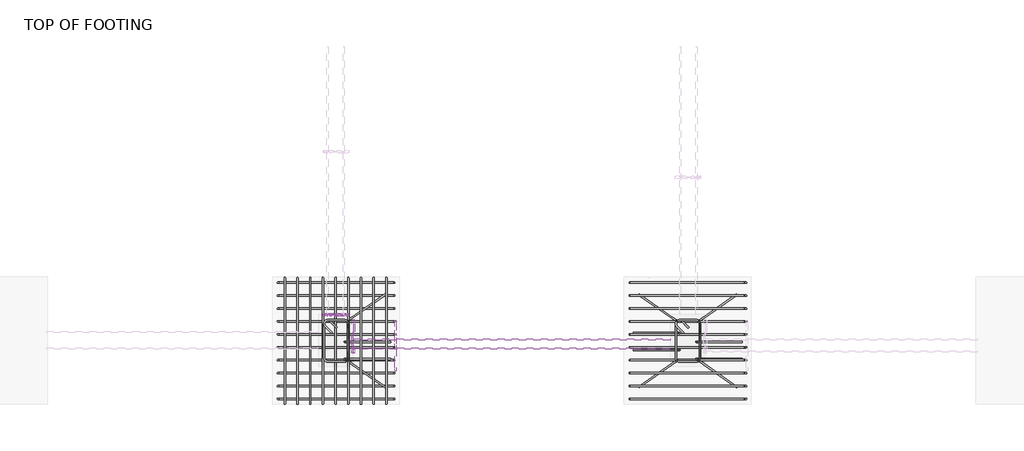
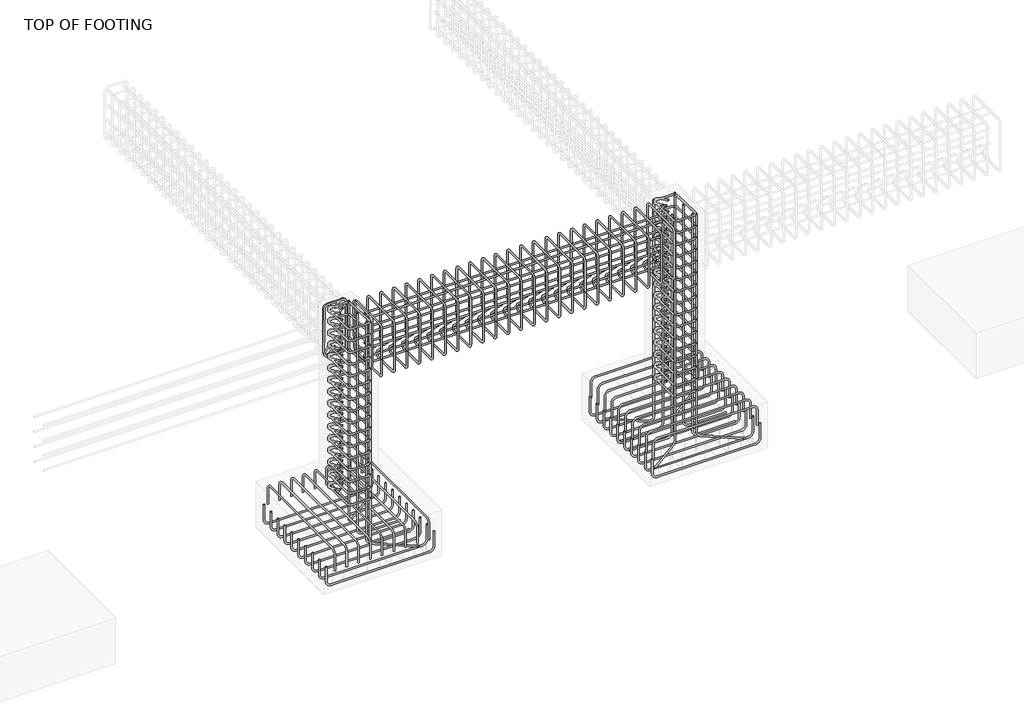
# One storey, part 3 of 18: 21 reinforcing bars.
"""IFC4 building model written with IfcOpenShell, lengths in millimetres."""

from ifc_helpers import new_model, si_unit, point, frame, origin, place, context, project, spatial, polyline, circle_curve, trimmed, segment, composite_curve, source, transform, mapped, element, save
from ifc_brep_helpers import swept_disk

model = new_model("IFC4")

# Units and contexts
model_context = context("Model", 3, world=origin())
ifc_project = project(units=[si_unit("LENGTHUNIT", "METRE", prefix="MILLI")], contexts=[model_context])

# Site, building, storey
site = spatial("IfcSite", under=ifc_project)
building = spatial("IfcBuilding", under=site)
storey = spatial("IfcBuildingStorey", under=building, Name="TOP OF FOOTING", Elevation=-1828.8)

# Reinforcing bars
placement = place(None, origin())
reinforcing_bar_shape = source(origin(), model_context, "Body", "SolidModel", [
    swept_disk(composite_curve([segment(polyline([(-7988.6954038, 5770.3841028, -1782.45), (-8044.4389667, 5826.1276657, -1782.45)]), True, "CONTINUOUS"), segment(trimmed(circle_curve(frame((-8066.6067643, 5803.9598681, -1782.45), z_axis=(0.0, 0.0, 1.0), x_axis=(22.167797600000085, 22.167797600000085, 0.0)), 31.35), [point((-8044.4389667, 5826.1276657, -1782.45))], [point((-8097.9567643, 5803.9598681, -1782.45))], True, "CARTESIAN"), True, "CONTINUOUS"), segment(polyline([(-8097.9567643, 5803.9598681, -1782.45), (-8097.9567643, 5509.3598681, -1782.45)]), True, "CONTINUOUS"), segment(trimmed(circle_curve(frame((-8066.6067643, 5509.3598681, -1782.45), z_axis=(0.0, 0.0, 1.0), x_axis=(-31.350000000000364, 0.0, 0.0)), 31.35), [point((-8097.9567643, 5509.3598681, -1782.45))], [point((-8066.6067643, 5478.0098681, -1782.45))], True, "CARTESIAN"), True, "CONTINUOUS"), segment(polyline([(-8066.6067643, 5478.0098681, -1782.45), (-7922.0067643, 5478.0098681, -1782.45)]), True, "CONTINUOUS"), segment(trimmed(circle_curve(frame((-7922.0067643, 5509.3400831, -1783.5636125), z_axis=(0.0, 0.03552192833448201, 0.9993688971583016), x_axis=(0.0, -31.330214999999953, 1.1136125000000447)), 31.35), [point((-7922.0067643, 5478.0098681, -1782.45))], [point((-7890.6567643, 5509.3400831, -1783.5636125))], True, "CARTESIAN"), True, "CONTINUOUS"), segment(polyline([(-7890.6567643, 5509.3400831, -1783.5636125), (-7890.6567643, 5803.9796532, -1794.0363875)]), True, "CONTINUOUS"), segment(trimmed(circle_curve(frame((-7922.0067643, 5803.9796532, -1794.0363875), z_axis=(0.0, 0.03552192833448201, 0.9993688971583016), x_axis=(31.350000000000364, 0.0, 0.0)), 31.35), [point((-7890.6567643, 5803.9796532, -1794.0363875))], [point((-7922.0067643, 5835.3098681, -1795.15))], True, "CARTESIAN"), True, "CONTINUOUS"), segment(polyline([(-7922.0067643, 5835.3098681, -1795.15), (-8066.6067643, 5835.3098681, -1795.15)]), True, "CONTINUOUS"), segment(trimmed(circle_curve(frame((-8066.6067643, 5803.9598681, -1795.15), z_axis=(0.0, 0.0, 1.0), x_axis=(0.0, 31.350000000000364, 0.0)), 31.35), [point((-8066.6067643, 5835.3098681, -1795.15))], [point((-8088.7745619, 5781.7920705, -1795.15))], True, "CARTESIAN"), True, "CONTINUOUS"), segment(polyline([(-8088.7745619, 5781.7920705, -1795.15), (-8033.030999, 5726.0485076, -1795.15)]), True, "CONTINUOUS")], self_intersect=False), 6.35),
])
element("IfcReinforcingBar", 1, at=placement, inside=storey, context=model_context, shape_type="MappedRepresentation", body=[
    mapped(reinforcing_bar_shape, transform((0.0, 0.0, 0.0), x_axis=(1.0, 0.0, 0.0), y_axis=(0.0, 1.0, 0.0), z_axis=(0.0, 0.0, 1.0))),
    mapped(reinforcing_bar_shape, transform((0.0, 0.0, 116.0092918), x_axis=(1.0, 0.0, 0.0), y_axis=(0.0, 1.0, 0.0), z_axis=(0.0, 0.0, 1.0))),
    mapped(reinforcing_bar_shape, transform((0.0, 0.0, 232.0185836), x_axis=(1.0, 0.0, 0.0), y_axis=(0.0, 1.0, 0.0), z_axis=(0.0, 0.0, 1.0))),
    mapped(reinforcing_bar_shape, transform((0.0, 0.0, 348.0278755), x_axis=(1.0, 0.0, 0.0), y_axis=(0.0, 1.0, 0.0), z_axis=(0.0, 0.0, 1.0))),
    mapped(reinforcing_bar_shape, transform((0.0, 0.0, 464.0371673), x_axis=(1.0, 0.0, 0.0), y_axis=(0.0, 1.0, 0.0), z_axis=(0.0, 0.0, 1.0))),
    mapped(reinforcing_bar_shape, transform((0.0, 0.0, 580.0464591), x_axis=(1.0, 0.0, 0.0), y_axis=(0.0, 1.0, 0.0), z_axis=(0.0, 0.0, 1.0))),
    mapped(reinforcing_bar_shape, transform((0.0, 0.0, 696.0557509), x_axis=(1.0, 0.0, 0.0), y_axis=(0.0, 1.0, 0.0), z_axis=(0.0, 0.0, 1.0))),
    mapped(reinforcing_bar_shape, transform((0.0, 0.0, 812.0650428), x_axis=(1.0, 0.0, 0.0), y_axis=(0.0, 1.0, 0.0), z_axis=(0.0, 0.0, 1.0))),
    mapped(reinforcing_bar_shape, transform((0.0, 0.0, 928.0743346), x_axis=(1.0, 0.0, 0.0), y_axis=(0.0, 1.0, 0.0), z_axis=(0.0, 0.0, 1.0))),
    mapped(reinforcing_bar_shape, transform((0.0, 0.0, 1044.0836264), x_axis=(1.0, 0.0, 0.0), y_axis=(0.0, 1.0, 0.0), z_axis=(0.0, 0.0, 1.0))),
    mapped(reinforcing_bar_shape, transform((0.0, 0.0, 1160.0929182), x_axis=(1.0, 0.0, 0.0), y_axis=(0.0, 1.0, 0.0), z_axis=(0.0, 0.0, 1.0))),
    mapped(reinforcing_bar_shape, transform((0.0, 0.0, 1276.1022101), x_axis=(1.0, 0.0, 0.0), y_axis=(0.0, 1.0, 0.0), z_axis=(0.0, 0.0, 1.0))),
    mapped(reinforcing_bar_shape, transform((0.0, 0.0, 1392.1115019), x_axis=(1.0, 0.0, 0.0), y_axis=(0.0, 1.0, 0.0), z_axis=(0.0, 0.0, 1.0))),
    mapped(reinforcing_bar_shape, transform((0.0, 0.0, 1508.1207937), x_axis=(1.0, 0.0, 0.0), y_axis=(0.0, 1.0, 0.0), z_axis=(0.0, 0.0, 1.0))),
    mapped(reinforcing_bar_shape, transform((0.0, 0.0, 1624.1300855), x_axis=(1.0, 0.0, 0.0), y_axis=(0.0, 1.0, 0.0), z_axis=(0.0, 0.0, 1.0))),
    mapped(reinforcing_bar_shape, transform((0.0, 0.0, 1740.1393774), x_axis=(1.0, 0.0, 0.0), y_axis=(0.0, 1.0, 0.0), z_axis=(0.0, 0.0, 1.0))),
])
element("IfcReinforcingBar", 2, at=placement, inside=storey, context=model_context, shape_type="SolidModel", body=[
    swept_disk(composite_curve([segment(polyline([(-7895.6275643, 5830.3098681, -40.0), (-7895.6275643, 5830.3098681, -2185.2530621)]), True, "CONTINUOUS"), segment(trimmed(circle_curve(frame((-7857.6598671, 5856.895136, -2185.2530621), z_axis=(0.5735764363510552, -0.8191520442889855, 0.0), x_axis=(-37.96769719999975, -26.585267899999963, 0.0)), 46.35), [point((-7895.6275643, 5830.3098681, -2185.2530621))], [point((-7857.6598671, 5856.895136, -2231.6030621))], True, "CARTESIAN"), True, "CONTINUOUS"), segment(polyline([(-7857.6598671, 5856.895136, -2231.6030621), (-7569.9927964, 6058.3217874, -2231.6030621)]), True, "CONTINUOUS")], self_intersect=False), 6.35),
])
element("IfcReinforcingBar", 3, at=placement, inside=storey, context=model_context, shape_type="SolidModel", body=[
    swept_disk(composite_curve([segment(polyline([(-7895.6275643, 5483.0098681, -40.0), (-7895.6275643, 5483.0098681, -2185.2530621)]), True, "CONTINUOUS"), segment(trimmed(circle_curve(frame((-7857.6598671, 5456.4246003, -2185.2530621), z_axis=(-0.5735764363510997, -0.8191520442889543, 0.0), x_axis=(-37.96769719999975, 26.58526780000011, 0.0)), 46.35), [point((-7895.6275643, 5483.0098681, -2185.2530621))], [point((-7857.6598671, 5456.4246003, -2231.6030621))], True, "CARTESIAN"), True, "CONTINUOUS"), segment(polyline([(-7857.6598671, 5456.4246003, -2231.6030621), (-7569.9927964, 5254.9979489, -2231.6030621)]), True, "CONTINUOUS")], self_intersect=False), 6.35),
])
reinforcing_bar_2_shape = source(origin(), model_context, "Body", "SolidModel", [
    swept_disk(composite_curve([segment(polyline([(-7920.6275643, 5499.8477614, -40.0), (-7920.6275643, 5499.8477614, -2185.2530621)]), True, "CONTINUOUS"), segment(trimmed(circle_curve(frame((-7874.2775643, 5499.8477614, -2185.2530621), z_axis=(0.0, -1.0, 0.0), x_axis=(-46.349999999999454, 0.0, 0.0)), 46.35), [point((-7920.6275643, 5499.8477614, -2185.2530621))], [point((-7874.2775643, 5499.8477614, -2231.6030621))], True, "CARTESIAN"), True, "CONTINUOUS"), segment(polyline([(-7874.2775643, 5499.8477614, -2231.6030621), (-7523.1009144, 5499.8477614, -2231.6030621)]), True, "CONTINUOUS")], self_intersect=False), 6.35),
])
element("IfcReinforcingBar", 4, at=placement, inside=storey, context=model_context, shape_type="MappedRepresentation", body=[
    mapped(reinforcing_bar_2_shape, transform((0.0, 0.0, 0.0), x_axis=(1.0, 0.0, 0.0), y_axis=(0.0, 1.0, 0.0), z_axis=(0.0, 0.0, 1.0))),
    mapped(reinforcing_bar_2_shape, transform((0.0, 148.3194112, 0.0), x_axis=(1.0, 0.0, 0.0), y_axis=(0.0, 1.0, 0.0), z_axis=(0.0, 0.0, 1.0))),
])
reinforcing_bar_3_shape = source(origin(), model_context, "Body", "SolidModel", [
    swept_disk(composite_curve([segment(polyline([(-5019.9859643, 5574.8477614, -40.0), (-5019.9859643, 5574.8477614, -2185.2530621)]), True, "CONTINUOUS"), segment(trimmed(circle_curve(frame((-5066.3359643, 5574.8477614, -2185.2530621), z_axis=(0.0, 1.0, 0.0), x_axis=(46.350000000000364, 0.0, 0.0)), 46.35), [point((-5019.9859643, 5574.8477614, -2185.2530621))], [point((-5066.3359643, 5574.8477614, -2231.6030621))], True, "CARTESIAN"), True, "CONTINUOUS"), segment(polyline([(-5066.3359643, 5574.8477614, -2231.6030621), (-5417.5126143, 5574.8477614, -2231.6030621)]), True, "CONTINUOUS")], self_intersect=False), 6.35),
])
element("IfcReinforcingBar", 5, at=placement, inside=storey, context=model_context, shape_type="MappedRepresentation", body=[
    mapped(reinforcing_bar_3_shape, transform((0.0, 0.0, 0.0), x_axis=(1.0, 0.0, 0.0), y_axis=(0.0, 1.0, 0.0), z_axis=(0.0, 0.0, 1.0))),
    mapped(reinforcing_bar_3_shape, transform((0.0, 148.3194112, 0.0), x_axis=(1.0, 0.0, 0.0), y_axis=(0.0, 1.0, 0.0), z_axis=(0.0, 0.0, 1.0))),
])
element("IfcReinforcingBar", 6, at=placement, inside=storey, context=model_context, shape_type="SolidModel", body=[
    swept_disk(composite_curve([segment(polyline([(-5044.9859643, 5830.3098681, -40.0), (-5044.9859643, 5830.3098681, -2185.2530621)]), True, "CONTINUOUS"), segment(trimmed(circle_curve(frame((-5082.9536616, 5856.895136, -2185.2530621), z_axis=(0.5735764363510552, 0.8191520442889856, 0.0), x_axis=(37.9676972999996, -26.585267899999963, 0.0)), 46.35), [point((-5044.9859643, 5830.3098681, -2185.2530621))], [point((-5082.9536616, 5856.895136, -2231.6030621))], True, "CARTESIAN"), True, "CONTINUOUS"), segment(polyline([(-5082.9536616, 5856.895136, -2231.6030621), (-5370.6207323, 6058.3217874, -2231.6030621)]), True, "CONTINUOUS")], self_intersect=False), 6.35),
])
reinforcing_bar_4_shape = source(origin(), model_context, "Body", "SolidModel", [
    swept_disk(composite_curve([segment(polyline([(-4940.6954038, 5770.3841028, -1782.45), (-4996.4389667, 5826.1276657, -1782.45)]), True, "CONTINUOUS"), segment(trimmed(circle_curve(frame((-5018.6067643, 5803.9598681, -1782.45), z_axis=(0.0, 0.0, 1.0), x_axis=(22.167797600000085, 22.167797600000085, 0.0)), 31.35), [point((-4996.4389667, 5826.1276657, -1782.45))], [point((-5049.9567643, 5803.9598681, -1782.45))], True, "CARTESIAN"), True, "CONTINUOUS"), segment(polyline([(-5049.9567643, 5803.9598681, -1782.45), (-5049.9567643, 5509.3598681, -1782.45)]), True, "CONTINUOUS"), segment(trimmed(circle_curve(frame((-5018.6067643, 5509.3598681, -1782.45), z_axis=(0.0, 0.0, 1.0), x_axis=(-31.350000000000364, 0.0, 0.0)), 31.35), [point((-5049.9567643, 5509.3598681, -1782.45))], [point((-5018.6067643, 5478.0098681, -1782.45))], True, "CARTESIAN"), True, "CONTINUOUS"), segment(polyline([(-5018.6067643, 5478.0098681, -1782.45), (-4874.0067643, 5478.0098681, -1782.45)]), True, "CONTINUOUS"), segment(trimmed(circle_curve(frame((-4874.0067643, 5509.3400831, -1783.5636125), z_axis=(0.0, 0.0355219283344819, 0.9993688971583016), x_axis=(0.0, -31.330214999999953, 1.1136125000000447)), 31.35), [point((-4874.0067643, 5478.0098681, -1782.45))], [point((-4842.6567643, 5509.3400831, -1783.5636125))], True, "CARTESIAN"), True, "CONTINUOUS"), segment(polyline([(-4842.6567643, 5509.3400831, -1783.5636125), (-4842.6567643, 5803.9796532, -1794.0363875)]), True, "CONTINUOUS"), segment(trimmed(circle_curve(frame((-4874.0067643, 5803.9796532, -1794.0363875), z_axis=(0.0, 0.0355219283344819, 0.9993688971583016), x_axis=(31.350000000000364, 0.0, 0.0)), 31.35), [point((-4842.6567643, 5803.9796532, -1794.0363875))], [point((-4874.0067643, 5835.3098681, -1795.15))], True, "CARTESIAN"), True, "CONTINUOUS"), segment(polyline([(-4874.0067643, 5835.3098681, -1795.15), (-5018.6067643, 5835.3098681, -1795.15)]), True, "CONTINUOUS"), segment(trimmed(circle_curve(frame((-5018.6067643, 5803.9598681, -1795.15), z_axis=(0.0, 0.0, 1.0), x_axis=(0.0, 31.350000000000364, 0.0)), 31.35), [point((-5018.6067643, 5835.3098681, -1795.15))], [point((-5040.7745619, 5781.7920705, -1795.15))], True, "CARTESIAN"), True, "CONTINUOUS"), segment(polyline([(-5040.7745619, 5781.7920705, -1795.15), (-4985.030999, 5726.0485076, -1795.15)]), True, "CONTINUOUS")], self_intersect=False), 6.35),
])
element("IfcReinforcingBar", 7, at=placement, inside=storey, context=model_context, shape_type="MappedRepresentation", body=[
    mapped(reinforcing_bar_4_shape, transform((0.0, 0.0, 0.0), x_axis=(1.0, 0.0, 0.0), y_axis=(0.0, 1.0, 0.0), z_axis=(0.0, 0.0, 1.0))),
    mapped(reinforcing_bar_4_shape, transform((0.0, 0.0, 116.0092918), x_axis=(1.0, 0.0, 0.0), y_axis=(0.0, 1.0, 0.0), z_axis=(0.0, 0.0, 1.0))),
    mapped(reinforcing_bar_4_shape, transform((0.0, 0.0, 232.0185836), x_axis=(1.0, 0.0, 0.0), y_axis=(0.0, 1.0, 0.0), z_axis=(0.0, 0.0, 1.0))),
    mapped(reinforcing_bar_4_shape, transform((0.0, 0.0, 348.0278755), x_axis=(1.0, 0.0, 0.0), y_axis=(0.0, 1.0, 0.0), z_axis=(0.0, 0.0, 1.0))),
    mapped(reinforcing_bar_4_shape, transform((0.0, 0.0, 464.0371673), x_axis=(1.0, 0.0, 0.0), y_axis=(0.0, 1.0, 0.0), z_axis=(0.0, 0.0, 1.0))),
    mapped(reinforcing_bar_4_shape, transform((0.0, 0.0, 580.0464591), x_axis=(1.0, 0.0, 0.0), y_axis=(0.0, 1.0, 0.0), z_axis=(0.0, 0.0, 1.0))),
    mapped(reinforcing_bar_4_shape, transform((0.0, 0.0, 696.0557509), x_axis=(1.0, 0.0, 0.0), y_axis=(0.0, 1.0, 0.0), z_axis=(0.0, 0.0, 1.0))),
    mapped(reinforcing_bar_4_shape, transform((0.0, 0.0, 812.0650428), x_axis=(1.0, 0.0, 0.0), y_axis=(0.0, 1.0, 0.0), z_axis=(0.0, 0.0, 1.0))),
    mapped(reinforcing_bar_4_shape, transform((0.0, 0.0, 928.0743346), x_axis=(1.0, 0.0, 0.0), y_axis=(0.0, 1.0, 0.0), z_axis=(0.0, 0.0, 1.0))),
    mapped(reinforcing_bar_4_shape, transform((0.0, 0.0, 1044.0836264), x_axis=(1.0, 0.0, 0.0), y_axis=(0.0, 1.0, 0.0), z_axis=(0.0, 0.0, 1.0))),
    mapped(reinforcing_bar_4_shape, transform((0.0, 0.0, 1160.0929182), x_axis=(1.0, 0.0, 0.0), y_axis=(0.0, 1.0, 0.0), z_axis=(0.0, 0.0, 1.0))),
    mapped(reinforcing_bar_4_shape, transform((0.0, 0.0, 1276.1022101), x_axis=(1.0, 0.0, 0.0), y_axis=(0.0, 1.0, 0.0), z_axis=(0.0, 0.0, 1.0))),
    mapped(reinforcing_bar_4_shape, transform((0.0, 0.0, 1392.1115019), x_axis=(1.0, 0.0, 0.0), y_axis=(0.0, 1.0, 0.0), z_axis=(0.0, 0.0, 1.0))),
    mapped(reinforcing_bar_4_shape, transform((0.0, 0.0, 1508.1207937), x_axis=(1.0, 0.0, 0.0), y_axis=(0.0, 1.0, 0.0), z_axis=(0.0, 0.0, 1.0))),
    mapped(reinforcing_bar_4_shape, transform((0.0, 0.0, 1624.1300855), x_axis=(1.0, 0.0, 0.0), y_axis=(0.0, 1.0, 0.0), z_axis=(0.0, 0.0, 1.0))),
    mapped(reinforcing_bar_4_shape, transform((0.0, 0.0, 1740.1393774), x_axis=(1.0, 0.0, 0.0), y_axis=(0.0, 1.0, 0.0), z_axis=(0.0, 0.0, 1.0))),
])
element("IfcReinforcingBar", 8, at=placement, inside=storey, context=model_context, shape_type="SolidModel", body=[
    swept_disk(composite_curve([segment(polyline([(-4847.6275643, 5830.3098681, -40.0), (-4847.6275643, 5830.3098681, -2185.2530621)]), True, "CONTINUOUS"), segment(trimmed(circle_curve(frame((-4809.6598671, 5856.895136, -2185.2530621), z_axis=(0.5735764363510553, -0.8191520442889855, 0.0), x_axis=(-37.96769719999975, -26.585267899999963, 0.0)), 46.35), [point((-4847.6275643, 5830.3098681, -2185.2530621))], [point((-4809.6598671, 5856.895136, -2231.6030621))], True, "CARTESIAN"), True, "CONTINUOUS"), segment(polyline([(-4809.6598671, 5856.895136, -2231.6030621), (-4521.9927964, 6058.3217874, -2231.6030621)]), True, "CONTINUOUS")], self_intersect=False), 6.35),
])
element("IfcReinforcingBar", 9, at=placement, inside=storey, context=model_context, shape_type="SolidModel", body=[
    swept_disk(composite_curve([segment(polyline([(-5044.9859643, 5483.0098681, -40.0), (-5044.9859643, 5483.0098681, -2185.2530621)]), True, "CONTINUOUS"), segment(trimmed(circle_curve(frame((-5082.9536616, 5456.4246003, -2185.2530621), z_axis=(-0.5735764363510106, 0.8191520442890168, 0.0), x_axis=(37.9676972999996, 26.58526780000011, 0.0)), 46.35), [point((-5044.9859643, 5483.0098681, -2185.2530621))], [point((-5082.9536616, 5456.4246003, -2231.6030621))], True, "CARTESIAN"), True, "CONTINUOUS"), segment(polyline([(-5082.9536616, 5456.4246003, -2231.6030621), (-5370.6207323, 5254.9979489, -2231.6030621)]), True, "CONTINUOUS")], self_intersect=False), 6.35),
])
element("IfcReinforcingBar", 10, at=placement, inside=storey, context=model_context, shape_type="SolidModel", body=[
    swept_disk(composite_curve([segment(polyline([(-4847.6275643, 5483.0098681, -40.0), (-4847.6275643, 5483.0098681, -2185.2530621)]), True, "CONTINUOUS"), segment(trimmed(circle_curve(frame((-4809.6598671, 5456.4246003, -2185.2530621), z_axis=(-0.5735764363510997, -0.8191520442889544, 0.0), x_axis=(-37.96769719999975, 26.58526780000011, 0.0)), 46.35), [point((-4847.6275643, 5483.0098681, -2185.2530621))], [point((-4809.6598671, 5456.4246003, -2231.6030621))], True, "CARTESIAN"), True, "CONTINUOUS"), segment(polyline([(-4809.6598671, 5456.4246003, -2231.6030621), (-4521.9927964, 5254.9979489, -2231.6030621)]), True, "CONTINUOUS")], self_intersect=False), 6.35),
])
reinforcing_bar_5_shape = source(origin(), model_context, "Body", "SolidModel", [
    swept_disk(composite_curve([segment(polyline([(-4872.6275643, 5499.8477614, -40.0), (-4872.6275643, 5499.8477614, -2185.2530621)]), True, "CONTINUOUS"), segment(trimmed(circle_curve(frame((-4826.2775643, 5499.8477614, -2185.2530621), z_axis=(0.0, -1.0, 0.0), x_axis=(-46.349999999999454, 0.0, 0.0)), 46.35), [point((-4872.6275643, 5499.8477614, -2185.2530621))], [point((-4826.2775643, 5499.8477614, -2231.6030621))], True, "CARTESIAN"), True, "CONTINUOUS"), segment(polyline([(-4826.2775643, 5499.8477614, -2231.6030621), (-4475.1009144, 5499.8477614, -2231.6030621)]), True, "CONTINUOUS")], self_intersect=False), 6.35),
])
element("IfcReinforcingBar", 11, at=placement, inside=storey, context=model_context, shape_type="MappedRepresentation", body=[
    mapped(reinforcing_bar_5_shape, transform((0.0, 0.0, 0.0), x_axis=(1.0, 0.0, 0.0), y_axis=(0.0, 1.0, 0.0), z_axis=(0.0, 0.0, 1.0))),
    mapped(reinforcing_bar_5_shape, transform((0.0, 148.3194112, 0.0), x_axis=(1.0, 0.0, 0.0), y_axis=(0.0, 1.0, 0.0), z_axis=(0.0, 0.0, 1.0))),
])
reinforcing_bar_6_shape = source(origin(), model_context, "Body", "SolidModel", [
    swept_disk(composite_curve([segment(polyline([(-4442.6567643, 6160.3098681, -2046.8654906), (-4442.6567643, 6160.3098681, -2194.1654906)]), True, "CONTINUOUS"), segment(trimmed(circle_curve(frame((-4489.0067643, 6160.3098681, -2194.1654906), z_axis=(0.0, 1.0, 0.0), x_axis=(46.350000000000364, 0.0, 0.0)), 46.35), [point((-4442.6567643, 6160.3098681, -2194.1654906))], [point((-4489.0067643, 6160.3098681, -2240.5154906))], True, "CARTESIAN"), True, "CONTINUOUS"), segment(polyline([(-4489.0067643, 6160.3098681, -2240.5154906), (-5403.6067643, 6160.3098681, -2240.5154906)]), True, "CONTINUOUS"), segment(trimmed(circle_curve(frame((-5403.6067643, 6160.3098681, -2194.1654906), z_axis=(0.0, 1.0, 0.0), x_axis=(0.0, 0.0, -46.34999999999991)), 46.35), [point((-5403.6067643, 6160.3098681, -2240.5154906))], [point((-5449.9567643, 6160.3098681, -2194.1654906))], True, "CARTESIAN"), True, "CONTINUOUS"), segment(polyline([(-5449.9567643, 6160.3098681, -2194.1654906), (-5449.9567643, 6160.3098681, -2046.8654906)]), True, "CONTINUOUS")], self_intersect=False), 6.35),
])
element("IfcReinforcingBar", 12, at=placement, inside=storey, context=model_context, shape_type="MappedRepresentation", body=[
    mapped(reinforcing_bar_6_shape, transform((0.0, 0.0, 0.0), x_axis=(1.0, 0.0, 0.0), y_axis=(0.0, 1.0, 0.0), z_axis=(0.0, 0.0, 1.0))),
    mapped(reinforcing_bar_6_shape, transform((0.0, -111.9222222, 0.0), x_axis=(1.0, 0.0, 0.0), y_axis=(0.0, 1.0, 0.0), z_axis=(0.0, 0.0, 1.0))),
    mapped(reinforcing_bar_6_shape, transform((0.0, -223.8444444, 0.0), x_axis=(1.0, 0.0, 0.0), y_axis=(0.0, 1.0, 0.0), z_axis=(0.0, 0.0, 1.0))),
    mapped(reinforcing_bar_6_shape, transform((0.0, -335.7666667, 0.0), x_axis=(1.0, 0.0, 0.0), y_axis=(0.0, 1.0, 0.0), z_axis=(0.0, 0.0, 1.0))),
    mapped(reinforcing_bar_6_shape, transform((0.0, -447.6888889, 0.0), x_axis=(1.0, 0.0, 0.0), y_axis=(0.0, 1.0, 0.0), z_axis=(0.0, 0.0, 1.0))),
    mapped(reinforcing_bar_6_shape, transform((0.0, -559.6111111, 0.0), x_axis=(1.0, 0.0, 0.0), y_axis=(0.0, 1.0, 0.0), z_axis=(0.0, 0.0, 1.0))),
    mapped(reinforcing_bar_6_shape, transform((0.0, -671.5333333, 0.0), x_axis=(1.0, 0.0, 0.0), y_axis=(0.0, 1.0, 0.0), z_axis=(0.0, 0.0, 1.0))),
    mapped(reinforcing_bar_6_shape, transform((0.0, -783.4555556, 0.0), x_axis=(1.0, 0.0, 0.0), y_axis=(0.0, 1.0, 0.0), z_axis=(0.0, 0.0, 1.0))),
    mapped(reinforcing_bar_6_shape, transform((0.0, -895.3777778, 0.0), x_axis=(1.0, 0.0, 0.0), y_axis=(0.0, 1.0, 0.0), z_axis=(0.0, 0.0, 1.0))),
    mapped(reinforcing_bar_6_shape, transform((0.0, -1007.3, 0.0), x_axis=(1.0, 0.0, 0.0), y_axis=(0.0, 1.0, 0.0), z_axis=(0.0, 0.0, 1.0))),
])
reinforcing_bar_7_shape = source(origin(), model_context, "Body", "SolidModel", [
    swept_disk(composite_curve([segment(polyline([(-5440.4399078, 6160.3098681, -2056.7800629), (-5440.4399078, 6160.3098681, -1909.4800629)]), True, "CONTINUOUS"), segment(trimmed(circle_curve(frame((-5394.0899078, 6160.3098681, -1909.4800629), z_axis=(0.0, 1.0, 0.0), x_axis=(-46.349999999999454, 0.0, 0.0)), 46.35), [point((-5440.4399078, 6160.3098681, -1909.4800629))], [point((-5394.0899078, 6160.3098681, -1863.1300629))], True, "CARTESIAN"), True, "CONTINUOUS"), segment(polyline([(-5394.0899078, 6160.3098681, -1863.1300629), (-4514.3320898, 6160.3098681, -1863.1300629)]), True, "CONTINUOUS"), segment(trimmed(circle_curve(frame((-4514.3320898, 6160.3098681, -1909.4800629), z_axis=(0.0, 1.0, 0.0), x_axis=(0.0, 0.0, 46.34999999999991)), 46.35), [point((-4514.3320898, 6160.3098681, -1863.1300629))], [point((-4467.9820898, 6160.3098681, -1909.4800629))], True, "CARTESIAN"), True, "CONTINUOUS"), segment(polyline([(-4467.9820898, 6160.3098681, -1909.4800629), (-4467.9820898, 6160.3098681, -2056.7800629)]), True, "CONTINUOUS")], self_intersect=False), 6.35),
])
element("IfcReinforcingBar", 13, at=placement, inside=storey, context=model_context, shape_type="MappedRepresentation", body=[
    mapped(reinforcing_bar_7_shape, transform((0.0, 0.0, 0.0), x_axis=(1.0, 0.0, 0.0), y_axis=(0.0, 1.0, 0.0), z_axis=(0.0, 0.0, 1.0))),
    mapped(reinforcing_bar_7_shape, transform((0.0, -111.9222222, 0.0), x_axis=(1.0, 0.0, 0.0), y_axis=(0.0, 1.0, 0.0), z_axis=(0.0, 0.0, 1.0))),
    mapped(reinforcing_bar_7_shape, transform((0.0, -223.8444444, 0.0), x_axis=(1.0, 0.0, 0.0), y_axis=(0.0, 1.0, 0.0), z_axis=(0.0, 0.0, 1.0))),
    mapped(reinforcing_bar_7_shape, transform((0.0, -335.7666667, 0.0), x_axis=(1.0, 0.0, 0.0), y_axis=(0.0, 1.0, 0.0), z_axis=(0.0, 0.0, 1.0))),
    mapped(reinforcing_bar_7_shape, transform((0.0, -447.6888889, 0.0), x_axis=(1.0, 0.0, 0.0), y_axis=(0.0, 1.0, 0.0), z_axis=(0.0, 0.0, 1.0))),
    mapped(reinforcing_bar_7_shape, transform((0.0, -559.6111111, 0.0), x_axis=(1.0, 0.0, 0.0), y_axis=(0.0, 1.0, 0.0), z_axis=(0.0, 0.0, 1.0))),
    mapped(reinforcing_bar_7_shape, transform((0.0, -671.5333333, 0.0), x_axis=(1.0, 0.0, 0.0), y_axis=(0.0, 1.0, 0.0), z_axis=(0.0, 0.0, 1.0))),
    mapped(reinforcing_bar_7_shape, transform((0.0, -783.4555556, 0.0), x_axis=(1.0, 0.0, 0.0), y_axis=(0.0, 1.0, 0.0), z_axis=(0.0, 0.0, 1.0))),
    mapped(reinforcing_bar_7_shape, transform((0.0, -895.3777778, 0.0), x_axis=(1.0, 0.0, 0.0), y_axis=(0.0, 1.0, 0.0), z_axis=(0.0, 0.0, 1.0))),
    mapped(reinforcing_bar_7_shape, transform((0.0, -1007.3, 0.0), x_axis=(1.0, 0.0, 0.0), y_axis=(0.0, 1.0, 0.0), z_axis=(0.0, 0.0, 1.0))),
])
reinforcing_bar_8_shape = source(origin(), model_context, "Body", "SolidModel", [
    swept_disk(composite_curve([segment(polyline([(-7490.6567643, 6160.3098681, -2046.8654906), (-7490.6567643, 6160.3098681, -2194.1654906)]), True, "CONTINUOUS"), segment(trimmed(circle_curve(frame((-7537.0067643, 6160.3098681, -2194.1654906), z_axis=(0.0, 1.0, 0.0), x_axis=(46.350000000000364, 0.0, 0.0)), 46.35), [point((-7490.6567643, 6160.3098681, -2194.1654906))], [point((-7537.0067643, 6160.3098681, -2240.5154906))], True, "CARTESIAN"), True, "CONTINUOUS"), segment(polyline([(-7537.0067643, 6160.3098681, -2240.5154906), (-8451.6067643, 6160.3098681, -2240.5154906)]), True, "CONTINUOUS"), segment(trimmed(circle_curve(frame((-8451.6067643, 6160.3098681, -2194.1654906), z_axis=(0.0, 1.0, 0.0), x_axis=(0.0, 0.0, -46.34999999999991)), 46.35), [point((-8451.6067643, 6160.3098681, -2240.5154906))], [point((-8497.9567643, 6160.3098681, -2194.1654906))], True, "CARTESIAN"), True, "CONTINUOUS"), segment(polyline([(-8497.9567643, 6160.3098681, -2194.1654906), (-8497.9567643, 6160.3098681, -2046.8654906)]), True, "CONTINUOUS")], self_intersect=False), 6.35),
])
element("IfcReinforcingBar", 14, at=placement, inside=storey, context=model_context, shape_type="MappedRepresentation", body=[
    mapped(reinforcing_bar_8_shape, transform((0.0, 0.0, 0.0), x_axis=(1.0, 0.0, 0.0), y_axis=(0.0, 1.0, 0.0), z_axis=(0.0, 0.0, 1.0))),
    mapped(reinforcing_bar_8_shape, transform((0.0, -111.9222222, 0.0), x_axis=(1.0, 0.0, 0.0), y_axis=(0.0, 1.0, 0.0), z_axis=(0.0, 0.0, 1.0))),
    mapped(reinforcing_bar_8_shape, transform((0.0, -223.8444444, 0.0), x_axis=(1.0, 0.0, 0.0), y_axis=(0.0, 1.0, 0.0), z_axis=(0.0, 0.0, 1.0))),
    mapped(reinforcing_bar_8_shape, transform((0.0, -335.7666667, 0.0), x_axis=(1.0, 0.0, 0.0), y_axis=(0.0, 1.0, 0.0), z_axis=(0.0, 0.0, 1.0))),
    mapped(reinforcing_bar_8_shape, transform((0.0, -447.6888889, 0.0), x_axis=(1.0, 0.0, 0.0), y_axis=(0.0, 1.0, 0.0), z_axis=(0.0, 0.0, 1.0))),
    mapped(reinforcing_bar_8_shape, transform((0.0, -559.6111111, 0.0), x_axis=(1.0, 0.0, 0.0), y_axis=(0.0, 1.0, 0.0), z_axis=(0.0, 0.0, 1.0))),
    mapped(reinforcing_bar_8_shape, transform((0.0, -671.5333333, 0.0), x_axis=(1.0, 0.0, 0.0), y_axis=(0.0, 1.0, 0.0), z_axis=(0.0, 0.0, 1.0))),
    mapped(reinforcing_bar_8_shape, transform((0.0, -783.4555556, 0.0), x_axis=(1.0, 0.0, 0.0), y_axis=(0.0, 1.0, 0.0), z_axis=(0.0, 0.0, 1.0))),
    mapped(reinforcing_bar_8_shape, transform((0.0, -895.3777778, 0.0), x_axis=(1.0, 0.0, 0.0), y_axis=(0.0, 1.0, 0.0), z_axis=(0.0, 0.0, 1.0))),
    mapped(reinforcing_bar_8_shape, transform((0.0, -1007.3, 0.0), x_axis=(1.0, 0.0, 0.0), y_axis=(0.0, 1.0, 0.0), z_axis=(0.0, 0.0, 1.0))),
])
reinforcing_bar_9_shape = source(origin(), model_context, "Body", "SolidModel", [
    swept_disk(composite_curve([segment(polyline([(-7559.1065918, 6200.3098681, -2080.1793981), (-7559.1065918, 6200.3098681, -1932.8793981)]), True, "CONTINUOUS"), segment(trimmed(circle_curve(frame((-7559.1065918, 6153.9598681, -1932.8793981), z_axis=(1.0, 0.0, 0.0), x_axis=(0.0, 46.350000000000364, 0.0)), 46.35), [point((-7559.1065918, 6200.3098681, -1932.8793981))], [point((-7559.1065918, 6153.9598681, -1886.5293981))], True, "CARTESIAN"), True, "CONTINUOUS"), segment(polyline([(-7559.1065918, 6153.9598681, -1886.5293981), (-7559.1065918, 5159.3598681, -1886.5293981)]), True, "CONTINUOUS"), segment(trimmed(circle_curve(frame((-7559.1065918, 5159.3598681, -1932.8793981), z_axis=(1.0, 0.0, 0.0), x_axis=(0.0, 0.0, 46.34999999999991)), 46.35), [point((-7559.1065918, 5159.3598681, -1886.5293981))], [point((-7559.1065918, 5113.0098681, -1932.8793981))], True, "CARTESIAN"), True, "CONTINUOUS"), segment(polyline([(-7559.1065918, 5113.0098681, -1932.8793981), (-7559.1065918, 5113.0098681, -2080.1793981)]), True, "CONTINUOUS")], self_intersect=False), 6.35),
])
element("IfcReinforcingBar", 15, at=placement, inside=storey, context=model_context, shape_type="MappedRepresentation", body=[
    mapped(reinforcing_bar_9_shape, transform((0.0, 0.0, 0.0), x_axis=(1.0, 0.0, 0.0), y_axis=(0.0, 1.0, 0.0), z_axis=(0.0, 0.0, 1.0))),
    mapped(reinforcing_bar_9_shape, transform((-109.9785589, 0.0, 0.0), x_axis=(1.0, 0.0, 0.0), y_axis=(0.0, 1.0, 0.0), z_axis=(0.0, 0.0, 1.0))),
    mapped(reinforcing_bar_9_shape, transform((-219.9571177, 0.0, 0.0), x_axis=(1.0, 0.0, 0.0), y_axis=(0.0, 1.0, 0.0), z_axis=(0.0, 0.0, 1.0))),
    mapped(reinforcing_bar_9_shape, transform((-329.9356766, 0.0, 0.0), x_axis=(1.0, 0.0, 0.0), y_axis=(0.0, 1.0, 0.0), z_axis=(0.0, 0.0, 1.0))),
    mapped(reinforcing_bar_9_shape, transform((-439.9142355, 0.0, 0.0), x_axis=(1.0, 0.0, 0.0), y_axis=(0.0, 1.0, 0.0), z_axis=(0.0, 0.0, 1.0))),
    mapped(reinforcing_bar_9_shape, transform((-549.8927943, 0.0, 0.0), x_axis=(1.0, 0.0, 0.0), y_axis=(0.0, 1.0, 0.0), z_axis=(0.0, 0.0, 1.0))),
    mapped(reinforcing_bar_9_shape, transform((-659.8713532, 0.0, 0.0), x_axis=(1.0, 0.0, 0.0), y_axis=(0.0, 1.0, 0.0), z_axis=(0.0, 0.0, 1.0))),
    mapped(reinforcing_bar_9_shape, transform((-769.8499121, 0.0, 0.0), x_axis=(1.0, 0.0, 0.0), y_axis=(0.0, 1.0, 0.0), z_axis=(0.0, 0.0, 1.0))),
    mapped(reinforcing_bar_9_shape, transform((-879.828471, 0.0, 0.0), x_axis=(1.0, 0.0, 0.0), y_axis=(0.0, 1.0, 0.0), z_axis=(0.0, 0.0, 1.0))),
])
element("IfcReinforcingBar", 16, at=placement, inside=storey, context=model_context, shape_type="SolidModel", body=[
    swept_disk(composite_curve([segment(polyline([(-7999.9181249, 5888.0098675, -111.2757654), (-7944.1745619, 5888.0098675, -55.5322024)]), True, "CONTINUOUS"), segment(trimmed(circle_curve(frame((-7922.0067643, 5888.0098675, -77.7), z_axis=(0.0, 1.0, 0.0), x_axis=(-22.167797600000085, 0.0, 22.1677976)), 31.35), [point((-7944.1745619, 5888.0098675, -55.5322024))], [point((-7890.6567643, 5888.0098675, -77.7))], True, "CARTESIAN"), True, "CONTINUOUS"), segment(polyline([(-7890.6567643, 5888.0098675, -77.7), (-7890.6567643, 5888.0098675, -522.3)]), True, "CONTINUOUS"), segment(trimmed(circle_curve(frame((-7922.0067643, 5888.0098675, -522.3), z_axis=(0.0, 1.0, 0.0), x_axis=(31.350000000000364, 0.0, 0.0)), 31.35), [point((-7890.6567643, 5888.0098675, -522.3))], [point((-7922.0067643, 5888.0098675, -553.65))], True, "CARTESIAN"), True, "CONTINUOUS"), segment(polyline([(-7922.0067643, 5888.0098675, -553.65), (-8066.6067643, 5888.0098675, -553.65)]), True, "CONTINUOUS"), segment(trimmed(circle_curve(frame((-8066.6067643, 5887.2252819, -522.3098193), z_axis=(0.0, 0.9996867842138424, 0.025026655153786322), x_axis=(0.0, 0.784585600000355, -31.34018070000002)), 31.35), [point((-8066.6067643, 5888.0098675, -553.65))], [point((-8097.9567643, 5887.2252819, -522.3098193))], True, "CARTESIAN"), True, "CONTINUOUS"), segment(polyline([(-8097.9567643, 5887.2252819, -522.3098193), (-8097.9567643, 5876.0944532, -77.6901807)]), True, "CONTINUOUS"), segment(trimmed(circle_curve(frame((-8066.6067643, 5876.0944532, -77.6901807), z_axis=(0.0, 0.9996867842138424, 0.025026655153786322), x_axis=(-31.350000000000364, 0.0, 0.0)), 31.35), [point((-8097.9567643, 5876.0944532, -77.6901807))], [point((-8066.6067643, 5875.3098675, -46.35))], True, "CARTESIAN"), True, "CONTINUOUS"), segment(polyline([(-8066.6067643, 5875.3098675, -46.35), (-7922.0067643, 5875.3098675, -46.35)]), True, "CONTINUOUS"), segment(trimmed(circle_curve(frame((-7922.0067643, 5875.3098675, -77.7), z_axis=(0.0, 1.0, 0.0), x_axis=(0.0, 0.0, 31.35)), 31.35), [point((-7922.0067643, 5875.3098675, -46.35))], [point((-7899.8389667, 5875.3098675, -99.8677976))], True, "CARTESIAN"), True, "CONTINUOUS"), segment(polyline([(-7899.8389667, 5875.3098675, -99.8677976), (-7955.5825297, 5875.3098675, -155.6113605)]), True, "CONTINUOUS")], self_intersect=False), 6.35),
])
element("IfcReinforcingBar", 17, at=placement, inside=storey, context=model_context, shape_type="SolidModel", body=[
    swept_disk(composite_curve([segment(polyline([(-7988.6954038, 5888.0098675, -488.7242346), (-8044.4389667, 5888.0098675, -544.4677976)]), True, "CONTINUOUS"), segment(trimmed(circle_curve(frame((-8066.6067643, 5888.0098675, -522.3), z_axis=(0.0, 1.0, 0.0), x_axis=(22.167797600000085, 0.0, -22.167797600000085)), 31.35), [point((-8044.4389667, 5888.0098675, -544.4677976))], [point((-8097.9567643, 5888.0098675, -522.3))], True, "CARTESIAN"), True, "CONTINUOUS"), segment(polyline([(-8097.9567643, 5888.0098675, -522.3), (-8097.9567643, 5888.0098675, -77.7)]), True, "CONTINUOUS"), segment(trimmed(circle_curve(frame((-8066.6067643, 5888.0098675, -77.7), z_axis=(0.0, 1.0, 0.0), x_axis=(-31.350000000000364, 0.0, 0.0)), 31.35), [point((-8097.9567643, 5888.0098675, -77.7))], [point((-8066.6067643, 5888.0098675, -46.35))], True, "CARTESIAN"), True, "CONTINUOUS"), segment(polyline([(-8066.6067643, 5888.0098675, -46.35), (-7922.0067643, 5888.0098675, -46.35)]), True, "CONTINUOUS"), segment(trimmed(circle_curve(frame((-7922.0067643, 5887.2252819, -77.6901807), z_axis=(0.0, 0.9996867842138424, -0.025026655153786322), x_axis=(0.0, 0.784585600000355, 31.340180699999998)), 31.35), [point((-7922.0067643, 5888.0098675, -46.35))], [point((-7890.6567643, 5887.2252819, -77.6901807))], True, "CARTESIAN"), True, "CONTINUOUS"), segment(polyline([(-7890.6567643, 5887.2252819, -77.6901807), (-7890.6567643, 5876.0944532, -522.3098193)]), True, "CONTINUOUS"), segment(trimmed(circle_curve(frame((-7922.0067643, 5876.0944532, -522.3098193), z_axis=(0.0, 0.9996867842138424, -0.025026655153786322), x_axis=(31.350000000000364, 0.0, 0.0)), 31.35), [point((-7890.6567643, 5876.0944532, -522.3098193))], [point((-7922.0067643, 5875.3098675, -553.65))], True, "CARTESIAN"), True, "CONTINUOUS"), segment(polyline([(-7922.0067643, 5875.3098675, -553.65), (-8066.6067643, 5875.3098675, -553.65)]), True, "CONTINUOUS"), segment(trimmed(circle_curve(frame((-8066.6067643, 5875.3098675, -522.3), z_axis=(0.0, 1.0, 0.0), x_axis=(0.0, 0.0, -31.350000000000023)), 31.35), [point((-8066.6067643, 5875.3098675, -553.65))], [point((-8088.7745619, 5875.3098675, -500.1322024))], True, "CARTESIAN"), True, "CONTINUOUS"), segment(polyline([(-8088.7745619, 5875.3098675, -500.1322024), (-8033.030999, 5875.3098675, -444.3886395)]), True, "CONTINUOUS")], self_intersect=False), 6.35),
])
element("IfcReinforcingBar", 18, at=placement, inside=storey, context=model_context, shape_type="SolidModel", body=[
    swept_disk(composite_curve([segment(polyline([(-7837.9567643, 5662.2712287, -111.2757654), (-7837.9567643, 5606.5276657, -55.5322024)]), True, "CONTINUOUS"), segment(trimmed(circle_curve(frame((-7837.9567643, 5584.3598681, -77.7), z_axis=(1.0, 0.0, 0.0), x_axis=(0.0, 22.167797600000085, 22.1677976)), 31.35), [point((-7837.9567643, 5606.5276657, -55.5322024))], [point((-7837.9567643, 5553.0098681, -77.7))], True, "CARTESIAN"), True, "CONTINUOUS"), segment(polyline([(-7837.9567643, 5553.0098681, -77.7), (-7837.9567643, 5553.0098681, -522.3)]), True, "CONTINUOUS"), segment(trimmed(circle_curve(frame((-7837.9567643, 5584.3598681, -522.3), z_axis=(1.0, 0.0, 0.0), x_axis=(0.0, -31.350000000000364, 0.0)), 31.35), [point((-7837.9567643, 5553.0098681, -522.3))], [point((-7837.9567643, 5584.3598681, -553.65))], True, "CARTESIAN"), True, "CONTINUOUS"), segment(polyline([(-7837.9567643, 5584.3598681, -553.65), (-7837.9567643, 5803.9598681, -553.65)]), True, "CONTINUOUS"), segment(trimmed(circle_curve(frame((-7838.74135, 5803.9598681, -522.3098193), z_axis=(0.9996867842138424, 0.0, 0.02502665515378632), x_axis=(0.784585700000207, 0.0, -31.34018070000002)), 31.35), [point((-7837.9567643, 5803.9598681, -553.65))], [point((-7838.74135, 5835.3098681, -522.3098193))], True, "CARTESIAN"), True, "CONTINUOUS"), segment(polyline([(-7838.74135, 5835.3098681, -522.3098193), (-7849.8721787, 5835.3098681, -77.6901807)]), True, "CONTINUOUS"), segment(trimmed(circle_curve(frame((-7849.8721787, 5803.9598681, -77.6901807), z_axis=(0.9996867842138424, 0.0, 0.02502665515378632), x_axis=(0.0, 31.350000000000364, 0.0)), 31.35), [point((-7849.8721787, 5835.3098681, -77.6901807))], [point((-7850.6567643, 5803.9598681, -46.35))], True, "CARTESIAN"), True, "CONTINUOUS"), segment(polyline([(-7850.6567643, 5803.9598681, -46.35), (-7850.6567643, 5584.3598681, -46.35)]), True, "CONTINUOUS"), segment(trimmed(circle_curve(frame((-7850.6567643, 5584.3598681, -77.7), z_axis=(1.0, 0.0, 0.0), x_axis=(0.0, 0.0, 31.35)), 31.35), [point((-7850.6567643, 5584.3598681, -46.35))], [point((-7850.6567643, 5562.1920705, -99.8677976))], True, "CARTESIAN"), True, "CONTINUOUS"), segment(polyline([(-7850.6567643, 5562.1920705, -99.8677976), (-7850.6567643, 5617.9356335, -155.6113605)]), True, "CONTINUOUS")], self_intersect=False), 6.35),
])
reinforcing_bar_10_shape = source(origin(), model_context, "Body", "SolidModel", [
    swept_disk(composite_curve([segment(polyline([(-7837.9567643, 5721.0485076, -488.7242346), (-7837.9567643, 5776.7920705, -544.4677976)]), True, "CONTINUOUS"), segment(trimmed(circle_curve(frame((-7837.9567643, 5798.9598681, -522.3), z_axis=(1.0, 0.0, 0.0), x_axis=(0.0, -22.167797600000085, -22.167797600000085)), 31.35), [point((-7837.9567643, 5776.7920705, -544.4677976))], [point((-7837.9567643, 5830.3098681, -522.3))], True, "CARTESIAN"), True, "CONTINUOUS"), segment(polyline([(-7837.9567643, 5830.3098681, -522.3), (-7837.9567643, 5830.3098681, -77.7)]), True, "CONTINUOUS"), segment(trimmed(circle_curve(frame((-7837.9567643, 5798.9598681, -77.7), z_axis=(1.0, 0.0, 0.0), x_axis=(0.0, 31.350000000000364, 0.0)), 31.35), [point((-7837.9567643, 5830.3098681, -77.7))], [point((-7837.9567643, 5798.9598681, -46.35))], True, "CARTESIAN"), True, "CONTINUOUS"), segment(polyline([(-7837.9567643, 5798.9598681, -46.35), (-7837.9567643, 5429.3598681, -46.35)]), True, "CONTINUOUS"), segment(trimmed(circle_curve(frame((-7837.9567643, 5429.3598681, -77.7), z_axis=(1.0, 0.0, 0.0), x_axis=(0.0, 0.0, 31.35)), 31.35), [point((-7837.9567643, 5429.3598681, -46.35))], [point((-7837.9567643, 5398.0098681, -77.7))], True, "CARTESIAN"), True, "CONTINUOUS"), segment(polyline([(-7837.9567643, 5398.0098681, -77.7), (-7837.9567643, 5398.0098681, -522.3)]), True, "CONTINUOUS"), segment(trimmed(circle_curve(frame((-7837.9567643, 5429.3598681, -522.3), z_axis=(1.0, 0.0, 0.0), x_axis=(0.0, -31.350000000000364, 0.0)), 31.35), [point((-7837.9567643, 5398.0098681, -522.3))], [point((-7837.9567643, 5429.3598681, -553.65))], True, "CARTESIAN"), True, "CONTINUOUS"), segment(polyline([(-7837.9567643, 5429.3598681, -553.65), (-7837.9567643, 5648.9598681, -553.65)]), True, "CONTINUOUS"), segment(trimmed(circle_curve(frame((-7837.9567643, 5648.9598681, -522.3), z_axis=(1.0, 0.0, 0.0), x_axis=(0.0, 0.0, -31.350000000000023)), 31.35), [point((-7837.9567643, 5648.9598681, -553.65))], [point((-7837.9567643, 5671.1276657, -500.1322024))], True, "CARTESIAN"), True, "CONTINUOUS"), segment(polyline([(-7837.9567643, 5671.1276657, -500.1322024), (-7837.9567643, 5615.3841028, -444.3886395)]), True, "CONTINUOUS")], self_intersect=False), 6.35),
])
element("IfcReinforcingBar", 19, at=placement, inside=storey, context=model_context, shape_type="MappedRepresentation", body=[
    mapped(reinforcing_bar_10_shape, transform((0.0, 0.0, 0.0), x_axis=(1.0, 0.0, 0.0), y_axis=(0.0, 1.0, 0.0), z_axis=(0.0, 0.0, 1.0))),
    mapped(reinforcing_bar_10_shape, transform((118.926087, 0.0, 0.0), x_axis=(1.0, 0.0, 0.0), y_axis=(0.0, 1.0, 0.0), z_axis=(0.0, 0.0, 1.0))),
    mapped(reinforcing_bar_10_shape, transform((237.8521739, 0.0, 0.0), x_axis=(1.0, 0.0, 0.0), y_axis=(0.0, 1.0, 0.0), z_axis=(0.0, 0.0, 1.0))),
    mapped(reinforcing_bar_10_shape, transform((356.7782609, 0.0, 0.0), x_axis=(1.0, 0.0, 0.0), y_axis=(0.0, 1.0, 0.0), z_axis=(0.0, 0.0, 1.0))),
    mapped(reinforcing_bar_10_shape, transform((475.7043478, 0.0, 0.0), x_axis=(1.0, 0.0, 0.0), y_axis=(0.0, 1.0, 0.0), z_axis=(0.0, 0.0, 1.0))),
    mapped(reinforcing_bar_10_shape, transform((594.6304348, 0.0, 0.0), x_axis=(1.0, 0.0, 0.0), y_axis=(0.0, 1.0, 0.0), z_axis=(0.0, 0.0, 1.0))),
    mapped(reinforcing_bar_10_shape, transform((713.5565217, 0.0, 0.0), x_axis=(1.0, 0.0, 0.0), y_axis=(0.0, 1.0, 0.0), z_axis=(0.0, 0.0, 1.0))),
    mapped(reinforcing_bar_10_shape, transform((832.4826087, 0.0, 0.0), x_axis=(1.0, 0.0, 0.0), y_axis=(0.0, 1.0, 0.0), z_axis=(0.0, 0.0, 1.0))),
    mapped(reinforcing_bar_10_shape, transform((951.4086957, 0.0, 0.0), x_axis=(1.0, 0.0, 0.0), y_axis=(0.0, 1.0, 0.0), z_axis=(0.0, 0.0, 1.0))),
    mapped(reinforcing_bar_10_shape, transform((1070.3347826, 0.0, 0.0), x_axis=(1.0, 0.0, 0.0), y_axis=(0.0, 1.0, 0.0), z_axis=(0.0, 0.0, 1.0))),
    mapped(reinforcing_bar_10_shape, transform((1189.2608696, 0.0, 0.0), x_axis=(1.0, 0.0, 0.0), y_axis=(0.0, 1.0, 0.0), z_axis=(0.0, 0.0, 1.0))),
    mapped(reinforcing_bar_10_shape, transform((1308.1869565, 0.0, 0.0), x_axis=(1.0, 0.0, 0.0), y_axis=(0.0, 1.0, 0.0), z_axis=(0.0, 0.0, 1.0))),
    mapped(reinforcing_bar_10_shape, transform((1427.1130435, 0.0, 0.0), x_axis=(1.0, 0.0, 0.0), y_axis=(0.0, 1.0, 0.0), z_axis=(0.0, 0.0, 1.0))),
    mapped(reinforcing_bar_10_shape, transform((1546.0391304, 0.0, 0.0), x_axis=(1.0, 0.0, 0.0), y_axis=(0.0, 1.0, 0.0), z_axis=(0.0, 0.0, 1.0))),
    mapped(reinforcing_bar_10_shape, transform((1664.9652174, 0.0, 0.0), x_axis=(1.0, 0.0, 0.0), y_axis=(0.0, 1.0, 0.0), z_axis=(0.0, 0.0, 1.0))),
    mapped(reinforcing_bar_10_shape, transform((1783.8913043, 0.0, 0.0), x_axis=(1.0, 0.0, 0.0), y_axis=(0.0, 1.0, 0.0), z_axis=(0.0, 0.0, 1.0))),
    mapped(reinforcing_bar_10_shape, transform((1902.8173913, 0.0, 0.0), x_axis=(1.0, 0.0, 0.0), y_axis=(0.0, 1.0, 0.0), z_axis=(0.0, 0.0, 1.0))),
    mapped(reinforcing_bar_10_shape, transform((2021.7434783, 0.0, 0.0), x_axis=(1.0, 0.0, 0.0), y_axis=(0.0, 1.0, 0.0), z_axis=(0.0, 0.0, 1.0))),
    mapped(reinforcing_bar_10_shape, transform((2140.6695652, 0.0, 0.0), x_axis=(1.0, 0.0, 0.0), y_axis=(0.0, 1.0, 0.0), z_axis=(0.0, 0.0, 1.0))),
    mapped(reinforcing_bar_10_shape, transform((2259.5956522, 0.0, 0.0), x_axis=(1.0, 0.0, 0.0), y_axis=(0.0, 1.0, 0.0), z_axis=(0.0, 0.0, 1.0))),
    mapped(reinforcing_bar_10_shape, transform((2378.5217391, 0.0, 0.0), x_axis=(1.0, 0.0, 0.0), y_axis=(0.0, 1.0, 0.0), z_axis=(0.0, 0.0, 1.0))),
    mapped(reinforcing_bar_10_shape, transform((2497.4478261, 0.0, 0.0), x_axis=(1.0, 0.0, 0.0), y_axis=(0.0, 1.0, 0.0), z_axis=(0.0, 0.0, 1.0))),
    mapped(reinforcing_bar_10_shape, transform((2616.373913, 0.0, 0.0), x_axis=(1.0, 0.0, 0.0), y_axis=(0.0, 1.0, 0.0), z_axis=(0.0, 0.0, 1.0))),
    mapped(reinforcing_bar_10_shape, transform((2735.3, 0.0, 0.0), x_axis=(1.0, 0.0, 0.0), y_axis=(0.0, 1.0, 0.0), z_axis=(0.0, 0.0, 1.0))),
])
reinforcing_bar_11_shape = source(origin(), model_context, "Body", "SolidModel", [
    swept_disk(composite_curve([segment(polyline([(-7843.9117926, 5667.6098681, -522.3), (-5100.6053332, 5667.6098681, -522.3)]), True, "CONTINUOUS")], self_intersect=False), 6.35),
])
element("IfcReinforcingBar", 20, at=placement, inside=storey, context=model_context, shape_type="MappedRepresentation", body=[
    mapped(reinforcing_bar_11_shape, transform((0.0, 0.0, 0.0), x_axis=(1.0, 0.0, 0.0), y_axis=(0.0, 1.0, 0.0), z_axis=(0.0, 0.0, 1.0))),
    mapped(reinforcing_bar_11_shape, transform((0.0, 0.0, 146.4972976), x_axis=(1.0, 0.0, 0.0), y_axis=(0.0, 1.0, 0.0), z_axis=(0.0, 0.0, 1.0))),
    mapped(reinforcing_bar_11_shape, transform((0.0, 0.0, 292.9945952), x_axis=(1.0, 0.0, 0.0), y_axis=(0.0, 1.0, 0.0), z_axis=(0.0, 0.0, 1.0))),
    mapped(reinforcing_bar_11_shape, transform((0.0, 0.0, 439.4918929), x_axis=(1.0, 0.0, 0.0), y_axis=(0.0, 1.0, 0.0), z_axis=(0.0, 0.0, 1.0))),
])
reinforcing_bar_12_shape = source(origin(), model_context, "Body", "SolidModel", [
    swept_disk(composite_curve([segment(polyline([(-7839.2923997, 5590.7272016, -524.1097861), (-5106.6214141, 5590.7272016, -524.1097861)]), True, "CONTINUOUS")], self_intersect=False), 6.35),
])
element("IfcReinforcingBar", 21, at=placement, inside=storey, context=model_context, shape_type="MappedRepresentation", body=[
    mapped(reinforcing_bar_12_shape, transform((0.0, 0.0, 0.0), x_axis=(1.0, 0.0, 0.0), y_axis=(0.0, 1.0, 0.0), z_axis=(0.0, 0.0, 1.0))),
    mapped(reinforcing_bar_12_shape, transform((0.0, 0.0, 147.1005596), x_axis=(1.0, 0.0, 0.0), y_axis=(0.0, 1.0, 0.0), z_axis=(0.0, 0.0, 1.0))),
    mapped(reinforcing_bar_12_shape, transform((0.0, 0.0, 294.2011193), x_axis=(1.0, 0.0, 0.0), y_axis=(0.0, 1.0, 0.0), z_axis=(0.0, 0.0, 1.0))),
    mapped(reinforcing_bar_12_shape, transform((0.0, 0.0, 441.3016789), x_axis=(1.0, 0.0, 0.0), y_axis=(0.0, 1.0, 0.0), z_axis=(0.0, 0.0, 1.0))),
])

save(model, "model.ifc")

# Revit data of these elements
# Elements 1, 2, 3, 4, 5, 6, 7, 8, 9, 10, 11, 12, 13, 14, 15, 16, 17, 18, 19, 20, 21 (IfcReinforcingBar)
#   Phase Created = New Construction
